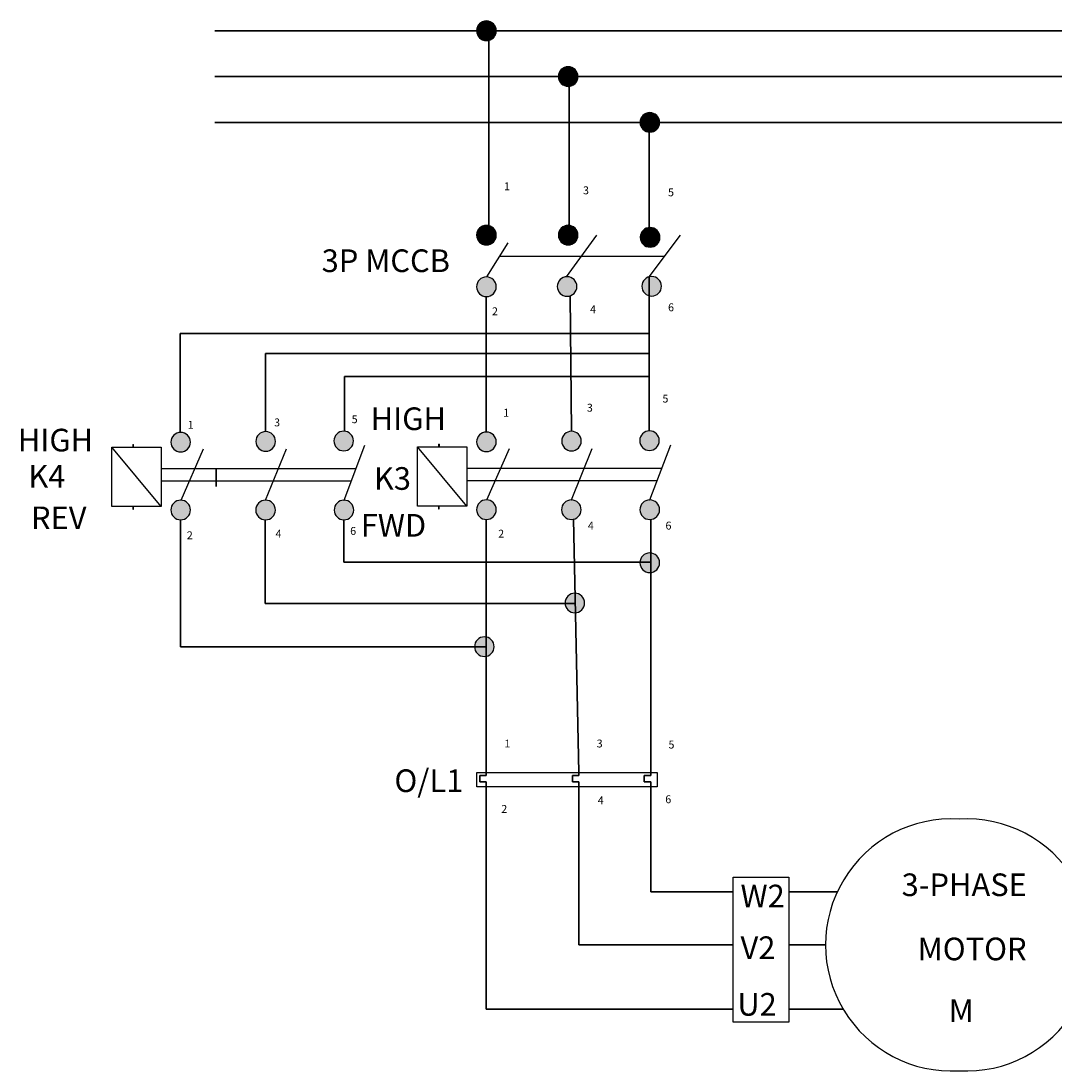
# Model space of a CAD drawing. Units: inches. Extents: x 5169 to 6773, y 5760 to 6563.
# Tile 1 of 2: x 5169 to 5959, y 5760 to 6563. Entities that reach past the tile are written whole.
import ezdxf

# ---------------------------------------------------------------- set-up
doc = ezdxf.new("R2010")
doc.units = ezdxf.units.IN
doc.header["$MEASUREMENT"] = 0
doc.layers.get('0').update_dxf_attribs({"color": 46})
for name, color, linetype, lineweight in [('E-ANNO-TEXT', 2, 'Continuous', 18), ('E-POWR-EQPM', 3, 'Continuous', 25), ('E-POWR-PATT', 8, 'Continuous', 18), ('E-POWR-WIRE', 7, 'Continuous', 35)]:
    doc.layers.add(name, color=color, linetype=linetype, lineweight=lineweight)
doc.styles.get("Standard").update_dxf_attribs({"font": 'arial.ttf'})

# ---------------------------------------------------------------- blocks, each defined once
blk = doc.blocks.new('CONTACTOR-COIL')
blk.add_line((37.69, 45.53), (0, 0))
blk.add_lwpolyline([(0, 0), (37.69, 0), (37.69, 45.53), (0, 45.53)], close=True)

msp = doc.modelspace()

# ---------------------------------------------------------------- hatches: boundary and pattern name
at = {"layer": 'E-POWR-PATT'}
h = msp.add_hatch(dxfattribs=at)
h.set_pattern_fill('ANSI31', color=256)
h.paths.add_polyline_path([(5517.59, 6555.12), (5532.59, 6555.12, 1)])
h.paths.add_polyline_path([(5532.59, 6555.12), (5517.59, 6555.12, 1)])
h.paths.add_polyline_path([(5580.08, 6520.12), (5595.08, 6520.12, 1)])
h.paths.add_polyline_path([(5595.08, 6520.12), (5580.08, 6520.12, 1)])
h.paths.add_polyline_path([(5642.56, 6485.12), (5657.56, 6485.12, 1)])
h.paths.add_polyline_path([(5657.56, 6485.12), (5642.56, 6485.12, 1)])
h = msp.add_hatch(dxfattribs=at)
h.set_pattern_fill('ANSI31', color=256)
h.paths.add_polyline_path([(5517.59, 6398.92, 1), (5532.59, 6398.92, 1)])
h.paths.add_polyline_path([(5595.08, 6398.94, 1), (5580.08, 6398.94, 1)])
h.paths.add_polyline_path([(5642.74, 6397.23, 1), (5657.74, 6397.23, 1)])
h = msp.add_hatch(color=256, dxfattribs=at)
h.dxf.hatch_style = 1
h.paths.add_polyline_path([(5532.59, 6359.49, 1), (5517.59, 6359.49, 1)])
h.paths.add_polyline_path([(5595.08, 6398.94, 1), (5580.08, 6398.94, 1)])
h.paths.add_polyline_path([(5517.59, 6398.92, 1), (5532.59, 6398.92, 1)])
h.paths.add_polyline_path([(5642.74, 6397.23, 1), (5657.74, 6397.23, 1)])
h.paths.add_polyline_path([(5594.25, 6359.66, 1), (5579.25, 6359.66, 1)])
h.paths.add_polyline_path([(5643.97, 6359.83, 1), (5658.97, 6359.83, 1)])
h = msp.add_hatch(color=256, dxfattribs=at)
h.dxf.hatch_style = 1
h.paths.add_polyline_path([(5298.72, 6240.68, 1), (5283.72, 6240.68, 1)])
h.paths.add_polyline_path([(5423.43, 6241.59, 1), (5408.43, 6241.59, 1)])
h = msp.add_hatch(color=256, dxfattribs=at)
h.dxf.hatch_style = 1
h.paths.add_polyline_path([(5348.76, 6241.25, 1), (5363.76, 6241.25, 1)])
h = msp.add_hatch(color=256, dxfattribs=at)
h.dxf.hatch_style = 1
h.paths.add_polyline_path([(5532.59, 6240.93, 1), (5517.59, 6240.93, 1)])
h.paths.add_polyline_path([(5582.63, 6241.5, 1), (5597.63, 6241.5, 1)])
h.paths.add_polyline_path([(5657.3, 6241.84, 1), (5642.3, 6241.84, 1)])
h = msp.add_hatch(color=256, dxfattribs=at)
h.dxf.hatch_style = 1
h.paths.add_polyline_path([(5255.2, 6238.78), (5254.61, 6238.78), (5254.61, 6236.92), (5255.2, 6236.92)])
h.paths.add_polyline_path([(5255.18, 6191.39), (5254.59, 6191.39), (5254.59, 6189.52), (5255.18, 6189.52)])
h = msp.add_hatch(color=256, dxfattribs=at)
h.dxf.hatch_style = 1
h.paths.add_polyline_path([(5489.07, 6239.03), (5488.48, 6239.03), (5488.48, 6237.16), (5489.07, 6237.16)])
h.paths.add_polyline_path([(5489.05, 6191.64), (5488.46, 6191.64), (5488.46, 6189.77), (5489.05, 6189.77)])
h = msp.add_hatch(color=256, dxfattribs=at)
h.dxf.hatch_style = 1
h.paths.add_polyline_path([(5283.72, 6188.82, 1), (5298.72, 6188.82, 1)])
h.paths.add_polyline_path([(5348.65, 6188.82), (5363.65, 6188.82, 0.996243)])
h = msp.add_hatch(color=256, dxfattribs=at)
h.dxf.hatch_style = 1
h.paths.add_polyline_path([(5517.59, 6189.07, 1), (5532.59, 6189.07, 1)])
h.paths.add_polyline_path([(5582.52, 6189.07), (5597.52, 6189.07, 0.996243)])
h = msp.add_hatch(color=256, dxfattribs=at)
h.dxf.hatch_style = 1
h.paths.add_polyline_path([(5597.52, 6189.04, 1), (5582.52, 6189.04, 1)])
h.paths.add_polyline_path([(5657.48, 6189.04, 0.407395), (5650.16, 6196.54), (5649.81, 6196.54, 0.407395), (5642.48, 6189.04, 1)])
h = msp.add_hatch(color=256, dxfattribs=at)
h.dxf.hatch_style = 1
h.paths.add_polyline_path([(5363.65, 6188.79, 1), (5348.65, 6188.79, 1)])
h.paths.add_polyline_path([(5423.61, 6188.8, 0.407395), (5416.28, 6196.29), (5415.93, 6196.29, 0.407395), (5408.61, 6188.8, 1)])
h = msp.add_hatch(color=256, dxfattribs=at)
h.dxf.hatch_style = 1
h.paths.add_polyline_path([(5524.97, 6084.34), (5515.97, 6084.34, 0.474651), (5524.97, 6076.99)])
h.paths.add_polyline_path([(5524.97, 6091.69, 0.474651), (5515.97, 6084.34), (5524.97, 6084.34)])
h.paths.add_polyline_path([(5524.97, 6091.69), (5524.97, 6084.34), (5524.97, 6076.99, 0.356253), (5530.97, 6084.34, 0.356253)])
h.paths.add_polyline_path([(5592.95, 6117.23), (5585.2, 6117.23, 0.410427), (5593.1, 6110.26)])
h.paths.add_polyline_path([(5592.78, 6125.24, 0.417716), (5585.19, 6117.74, 0.017058), (5585.2, 6117.23), (5592.95, 6117.23)])
h.paths.add_polyline_path([(5592.78, 6125.24), (5592.95, 6117.23), (5593.1, 6110.26, 0.398114), (5600.19, 6117.74, 0.41072)])
h.paths.add_polyline_path([(5650.79, 6148.87), (5642.49, 6148.87, 0.012478), (5642.48, 6148.49, 0.446102), (5650.79, 6141.04)])
h.paths.add_polyline_path([(5650.79, 6155.95, 0.431224), (5642.49, 6148.87), (5650.79, 6148.87)])
h.paths.add_polyline_path([(5650.79, 6155.95), (5650.79, 6148.87), (5650.79, 6141.04, 0.383028), (5657.48, 6148.49, 0.383028)])

# ---------------------------------------------------------------- linework, layer by layer
at = {"layer": 'E-POWR-EQPM'}
for p, q in [((5586.43, 6367.15), (5609.61, 6398.94)), ((5649.63, 6367.1), (5673.56, 6398.94)), ((5525.29, 6366.98), (5541.8, 6393.04)), ((5254.61, 6238.78), (5254.61, 6236.92)), ((5254.61, 6238.78), (5255.2, 6238.78)), ((5255.2, 6236.92), (5255.2, 6238.78)), ((5416.28, 6196.29), (5432.18, 6238.37)), ((5488.48, 6239.03), (5488.48, 6237.16)), ((5488.48, 6239.03), (5489.07, 6239.03)), ((5489.07, 6237.16), (5489.07, 6239.03)), ((5650.16, 6196.54), (5666.05, 6238.62)), ((5291.62, 6196.31), (5308.77, 6235.56)), ((5356.18, 6196.29), (5372.06, 6235.56)), ((5525.49, 6196.56), (5542.64, 6235.81)), ((5590.06, 6196.54), (5605.93, 6235.81)), ((5535.92, 6220.44), (5510.09, 6220.44)), ((5659.18, 6220.44), (5535.92, 6220.44)), ((5302.05, 6220.19), (5276.22, 6220.19)), ((5425.31, 6220.19), (5302.05, 6220.19)), ((5302.05, 6210.9), (5276.22, 6210.9)), ((5421.8, 6210.9), (5297.99, 6210.9)), ((5535.92, 6211.15), (5510.09, 6211.15)), ((5655.67, 6211.15), (5531.86, 6211.15)), ((5589.98, 6196.54), (5590.06, 6196.54)), ((5649.81, 6196.54), (5650.16, 6196.54)), ((5254.59, 6191.39), (5254.59, 6189.52)), ((5254.59, 6189.52), (5255.18, 6189.52)), ((5255.18, 6189.52), (5255.18, 6191.39)), ((5356.11, 6196.29), (5356.18, 6196.29)), ((5415.93, 6196.29), (5416.28, 6196.29)), ((5488.46, 6191.64), (5488.46, 6189.77)), ((5488.46, 6189.77), (5489.05, 6189.77)), ((5489.05, 6189.77), (5489.05, 6191.64))]:
    msp.add_line(p, q, dxfattribs=at)
for points in [[(5517.59, 6555.12, 1), (5532.59, 6555.12, 1)], [(5580.08, 6520.12, 1), (5595.08, 6520.12, 1)], [(5642.56, 6485.12, 1), (5657.56, 6485.12, 1)], [(5517.59, 6398.92, 1), (5532.59, 6398.92, 1)], [(5580.08, 6398.94, 1), (5595.08, 6398.94, 1)], [(5642.74, 6397.23, 1), (5657.74, 6397.23, 1)], [(5517.59, 6359.49, 1), (5532.59, 6359.49, 1)], [(5579.25, 6359.66, 1), (5594.25, 6359.66, 1)], [(5643.97, 6359.83, 1), (5658.97, 6359.83, 1)], [(5283.72, 6240.68, 1), (5298.72, 6240.68, 1)], [(5348.76, 6241.25, 1), (5363.76, 6241.25, 1)], [(5408.43, 6241.59, 1), (5423.43, 6241.59, 1)], [(5517.59, 6240.93, 1), (5532.59, 6240.93, 1)], [(5582.63, 6241.5, 1), (5597.63, 6241.5, 1)], [(5642.3, 6241.84, 1), (5657.3, 6241.84, 1)], [(5283.72, 6188.82, 1), (5298.72, 6188.82, 1)], [(5517.59, 6189.07, 1), (5532.59, 6189.07, 1)], [(5582.52, 6189.04, 1), (5597.52, 6189.04, 1)], [(5642.48, 6189.04, 1), (5657.48, 6189.04, 1)], [(5348.65, 6188.79, 1), (5363.65, 6188.79, 1)], [(5408.61, 6188.8, 1), (5423.61, 6188.8, 1)], [(5642.48, 6148.49, 1), (5657.48, 6148.49, 1)], [(5585.19, 6117.74, 1), (5600.19, 6117.74, 1)], [(5515.97, 6084.34, 1), (5530.97, 6084.34, 1)]]:
    msp.add_lwpolyline(points, format="xyb", close=True, dxfattribs=at)
for points in [[(5517.69, 5988.19), (5655.53, 5988.19), (5655.53, 5977.13), (5517.69, 5977.13)], [(5713.8, 5908.17), (5756.27, 5908.17), (5756.27, 5797.38), (5713.8, 5797.38)]]:
    msp.add_lwpolyline(points, close=True, dxfattribs=at)
for centre, start, end in [((5880.8, 5856.37), 86.60656, 273.39344), ((5892.21, 5856.37), 266.60656, 93.39344)]:
    msp.add_arc(centre, 96.38, start, end, dxfattribs=at)
at = {"layer": 'E-POWR-WIRE'}
for p, q in [((5317.39, 6555.12), (6439, 6555.12)), ((5526.89, 6547.84), (5526.89, 6406.2)), ((5317.39, 6520.12), (6438.76, 6520.12)), ((5588.34, 6512.66), (5588.34, 6406.4)), ((5317.39, 6485.12), (6439.26, 6485.12)), ((5649.63, 6477.63), (5649.63, 6404.46)), ((5649.63, 6404.46), (5649.63, 6389.76)), ((5661.38, 6382.73), (5535.24, 6382.7)), ((5649.63, 6367.1), (5649.63, 6249.34)), ((5524.97, 6351.99), (5524.97, 6248.43)), ((5589.02, 6352.51), (5590.09, 6249)), ((5290.91, 6248.18), (5290.91, 6323.73)), ((5290.91, 6323.73), (5318.35, 6323.73)), ((5649.63, 6323.73), (5318.35, 6323.73)), ((5649.63, 6308.43), (5356.22, 6308.43)), ((5356.22, 6308.43), (5356.22, 6248.75)), ((5649.63, 6290.9), (5416.47, 6290.9)), ((5416.47, 6249.07), (5416.47, 6290.9)), ((5318.35, 6220.19), (5318.35, 6206.72)), ((5291.11, 6181.32), (5291.11, 6084.34)), ((5355.89, 6181.3), (5355.89, 6117.23)), ((5416.06, 6181.3), (5416.06, 6148.87)), ((5524.97, 6181.57), (5524.97, 5988.19)), ((5591.55, 6181.7), (5595.75, 5988.19)), ((5650.79, 6181.59), (5650.79, 6031.06)), ((5416.06, 6148.87), (5650.79, 6148.87)), ((5355.89, 6117.23), (5592.95, 6117.23)), ((5291.11, 6084.34), (5524.97, 6084.34)), ((5650.79, 6031.06), (5650.79, 5988.19)), ((5524.97, 5985.99), (5524.97, 5988.19)), ((5595.79, 5985.99), (5595.75, 5988.19)), ((5650.79, 5988.19), (5650.79, 5985.99)), ((5524.97, 5985.99), (5519.97, 5985.99)), ((5519.97, 5985.99), (5519.97, 5980.99)), ((5519.97, 5980.99), (5524.97, 5980.99)), ((5524.97, 5980.99), (5524.97, 5977.13)), ((5595.79, 5985.99), (5590.79, 5985.99)), ((5590.79, 5985.99), (5590.79, 5980.99)), ((5590.79, 5980.99), (5595.79, 5980.99)), ((5595.79, 5980.99), (5595.79, 5977.13)), ((5650.79, 5985.99), (5645.79, 5985.99)), ((5645.79, 5985.99), (5645.79, 5980.99)), ((5645.79, 5980.99), (5650.79, 5980.99)), ((5650.79, 5980.99), (5650.79, 5977.13)), ((5524.97, 5977.13), (5524.97, 5807.35)), ((5595.79, 5977.13), (5595.79, 5856.37)), ((5650.79, 5977.13), (5650.79, 5897.03)), ((5650.79, 5897.03), (5713.8, 5897.03)), ((5756.27, 5897.03), (5793.42, 5897.03)), ((5595.79, 5856.37), (5713.8, 5856.37)), ((5756.27, 5856.37), (5784.42, 5856.37)), ((5524.97, 5807.35), (5713.8, 5807.35)), ((5756.27, 5807.35), (5797.82, 5807.35))]:
    msp.add_line(p, q, dxfattribs=at)

# ---------------------------------------------------------------- block references
at = {"layer": 'E-POWR-EQPM', "extrusion": (0, 0, -1), "zscale": -1, "rotation": 180}
for p in [(-5238.53, 6236.92), (-5472.4, 6237.16)]:
    msp.add_blockref('CONTACTOR-COIL', p, dxfattribs=at)

# ---------------------------------------------------------------- texts
at = {"layer": 'E-ANNO-TEXT'}
for s, height, p in [('1', 6.02, (5538.51, 6433.23)), ('3', 6.02, (5598.95, 6430.17)), ('5', 6.02, (5663.97, 6428.65)), ('3P MCCB', 17.303, (5399.07, 6370.72)), ('2', 6.02, (5529.33, 6337.69)), ('4', 6.02, (5604.3, 6339.22)), ('6', 6.02, (5663.97, 6340.75)), ('5', 6.02, (5659.71, 6270.93)), ('3', 6.02, (5601.89, 6264)), ('5', 6.02, (5422.02, 6255.16)), ('HIGH', 17.303, (5436.55, 6249.93)), ('1', 6.02, (5537.91, 6260.15)), ('1', 6.02, (5296.57, 6250.91)), ('3', 6.02, (5362.7, 6252.75)), ('HIGH', 17.303, (5166.73, 6233.6)), ('K4', 17.303, (5174.7, 6205.94)), ('K3', 17.303, (5439.01, 6204.25)), ('REV', 17.303, (5176.76, 6174.18)), ('FWD', 17.303, (5428.98, 6168.45)), ('2', 6.02, (5295.94, 6166.51)), ('4', 6.02, (5363.78, 6167.71)), ('6', 6.02, (5420.86, 6169.8)), ('2', 6.02, (5534.05, 6167.72)), ('4', 6.02, (5602.66, 6173.88)), ('6', 6.02, (5662.02, 6173.88)), ('1', 6.02, (5538.88, 6007.3)), ('3', 6.02, (5609.39, 6007.3)), ('5', 6.02, (5664.32, 6006.48)), ('O/L1', 17.303, (5454.7, 5973.23)), ('4', 6.02, (5610.21, 5963.88)), ('6', 6.02, (5661.86, 5964.7)), ('2', 6.02, (5536.42, 5957.33)), ('3-PHASE', 17.303, (5842.64, 5893.69)), ('W2', 17.303, (5719.41, 5885.08)), ('V2', 17.303, (5719.41, 5845.58)), ('MOTOR', 17.303, (5854.9, 5844.63)), ('U2', 17.303, (5716.96, 5802.28)), ('M', 17.3, (5878.63, 5797.55))]:
    msp.add_text(s, height=height, dxfattribs=at).set_placement(p)

doc.saveas('drawing.dxf')
